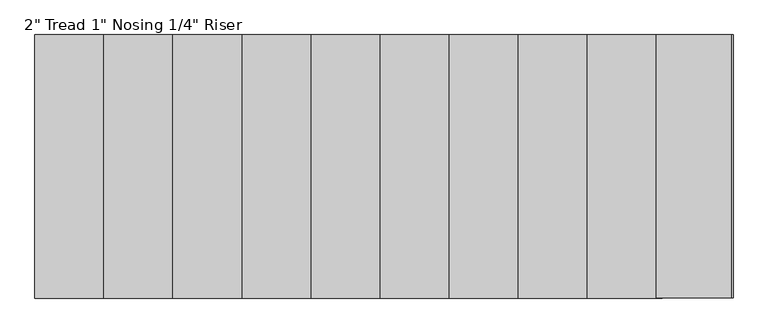
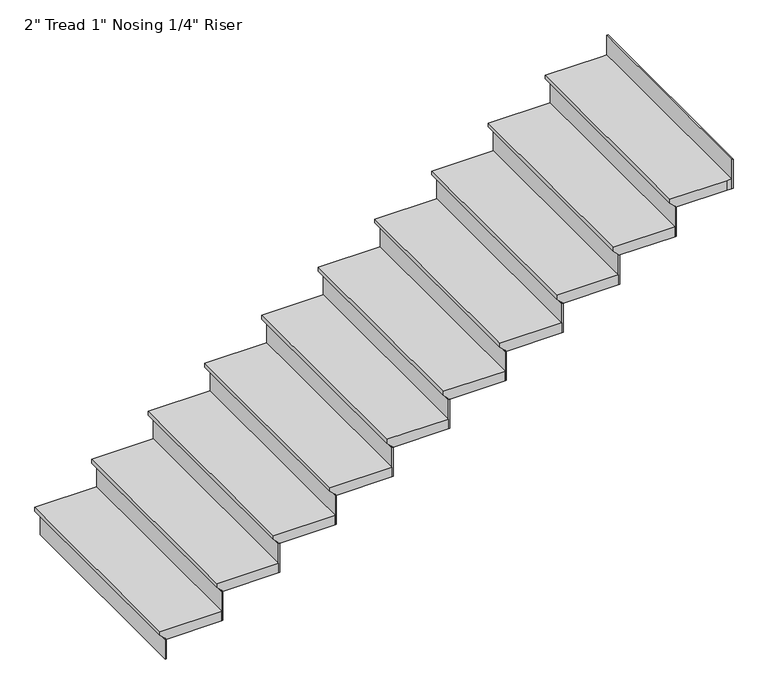
"""IFC4 building model written with IfcOpenShell, lengths in millimetres: stair flight geometry."""

from ifc_helpers import new_model, si_unit, origin, place, context, project, spatial, faceted_brep, source, transform, mapped, element, save


def stair_flight_2c29bb35(model_context):
    return source(origin(), model_context, "Body", "Brep", [
        faceted_brep([(-459.26646, -1849.1834702, 3181.35), (-459.26646, -1849.1834702, 3200.4), (-459.26646, -782.3834702, 3200.4), (-459.26646, -782.3834702, 3181.35), (-433.86646, -1849.1834702, 3155.95), (-433.86646, -782.3834702, 3155.95), (-154.46646, -1849.1834702, 3200.4), (-154.46646, -782.3834702, 3200.4), (-433.86646, -782.3834702, 3149.6), (-154.46646, -782.3834702, 3149.6), (-154.46646, -1849.1834702, 3149.6), (-433.86646, -1849.1834702, 3149.6)], [[[0, 1, 2, 3]], [[4, 0, 3, 5]], [[2, 1, 6, 7]], [[8, 9, 10, 11]], [[2, 7, 9, 8, 5, 3]], [[8, 11, 4, 5]], [[6, 1, 0, 4, 11, 10]], [[7, 6, 10, 9]]]),
        faceted_brep([(-433.86646, -1849.1834702, 3149.6), (-433.86646, -1849.1834702, 3048.0), (-427.51646, -1849.1834702, 3048.0), (-427.51646, -1849.1834702, 3149.6), (-433.86646, -782.3834702, 3149.6), (-427.51646, -782.3834702, 3149.6), (-427.51646, -782.3834702, 3048.0), (-433.86646, -782.3834702, 3048.0)], [[[0, 1, 2, 3]], [[4, 5, 6, 7]], [[1, 0, 4, 7]], [[2, 1, 7, 6]], [[3, 2, 6, 5]], [[0, 3, 5, 4]]]),
        faceted_brep([(-154.46646, -1849.1834702, 3302.0), (-154.46646, -1849.1834702, 3149.6), (-148.11646, -1849.1834702, 3149.6), (-148.11646, -1849.1834702, 3302.0), (-154.46646, -782.3834702, 3302.0), (-148.11646, -782.3834702, 3302.0), (-148.11646, -782.3834702, 3149.6), (-154.46646, -782.3834702, 3149.6)], [[[0, 1, 2, 3]], [[4, 5, 6, 7]], [[1, 0, 4, 7]], [[2, 1, 7, 6]], [[3, 2, 6, 5]], [[0, 3, 5, 4]]]),
        faceted_brep([(-179.86646, -782.3834702, 3352.8), (-179.86646, -1849.1834702, 3352.8), (124.93354, -1849.1834702, 3352.8), (124.93354, -782.3834702, 3352.8), (-154.46646, -782.3834702, 3302.0), (124.93354, -782.3834702, 3302.0), (124.93354, -1849.1834702, 3302.0), (-154.46646, -1849.1834702, 3302.0), (-154.46646, -782.3834702, 3308.35), (-179.86646, -782.3834702, 3333.75), (-154.46646, -1849.1834702, 3308.35), (-179.86646, -1849.1834702, 3333.75)], [[[0, 1, 2, 3]], [[4, 5, 6, 7]], [[0, 3, 5, 4, 8, 9]], [[4, 7, 10, 8]], [[2, 1, 11, 10, 7, 6]], [[3, 2, 6, 5]], [[11, 1, 0, 9]], [[10, 11, 9, 8]]]),
        faceted_brep([(124.93354, -1849.1834702, 3454.4), (124.93354, -1849.1834702, 3302.0), (131.28354, -1849.1834702, 3302.0), (131.28354, -1849.1834702, 3454.4), (124.93354, -782.3834702, 3454.4), (131.28354, -782.3834702, 3454.4), (131.28354, -782.3834702, 3302.0), (124.93354, -782.3834702, 3302.0)], [[[0, 1, 2, 3]], [[4, 5, 6, 7]], [[1, 0, 4, 7]], [[2, 1, 7, 6]], [[3, 2, 6, 5]], [[0, 3, 5, 4]]]),
        faceted_brep([(99.53354, -782.3834702, 3505.2), (99.53354, -1849.1834702, 3505.2), (404.33354, -1849.1834702, 3505.2), (404.33354, -782.3834702, 3505.2), (124.93354, -782.3834702, 3454.4), (404.33354, -782.3834702, 3454.4), (404.33354, -1849.1834702, 3454.4), (124.93354, -1849.1834702, 3454.4), (124.93354, -782.3834702, 3460.75), (99.53354, -782.3834702, 3486.15), (124.93354, -1849.1834702, 3460.75), (99.53354, -1849.1834702, 3486.15)], [[[0, 1, 2, 3]], [[4, 5, 6, 7]], [[0, 3, 5, 4, 8, 9]], [[4, 7, 10, 8]], [[2, 1, 11, 10, 7, 6]], [[3, 2, 6, 5]], [[11, 1, 0, 9]], [[10, 11, 9, 8]]]),
        faceted_brep([(404.33354, -1849.1834702, 3606.8), (404.33354, -1849.1834702, 3454.4), (410.68354, -1849.1834702, 3454.4), (410.68354, -1849.1834702, 3606.8), (404.33354, -782.3834702, 3606.8), (410.68354, -782.3834702, 3606.8), (410.68354, -782.3834702, 3454.4), (404.33354, -782.3834702, 3454.4)], [[[0, 1, 2, 3]], [[4, 5, 6, 7]], [[1, 0, 4, 7]], [[2, 1, 7, 6]], [[3, 2, 6, 5]], [[0, 3, 5, 4]]]),
        faceted_brep([(378.93354, -782.3834702, 3657.6), (378.93354, -1849.1834702, 3657.6), (683.73354, -1849.1834702, 3657.6), (683.73354, -782.3834702, 3657.6), (404.33354, -782.3834702, 3606.8), (683.73354, -782.3834702, 3606.8), (683.73354, -1849.1834702, 3606.8), (404.33354, -1849.1834702, 3606.8), (404.33354, -782.3834702, 3613.15), (378.93354, -782.3834702, 3638.55), (404.33354, -1849.1834702, 3613.15), (378.93354, -1849.1834702, 3638.55)], [[[0, 1, 2, 3]], [[4, 5, 6, 7]], [[0, 3, 5, 4, 8, 9]], [[4, 7, 10, 8]], [[2, 1, 11, 10, 7, 6]], [[3, 2, 6, 5]], [[11, 1, 0, 9]], [[10, 11, 9, 8]]]),
        faceted_brep([(683.73354, -1849.1834702, 3759.2), (683.73354, -1849.1834702, 3606.8), (690.08354, -1849.1834702, 3606.8), (690.08354, -1849.1834702, 3759.2), (683.73354, -782.3834702, 3759.2), (690.08354, -782.3834702, 3759.2), (690.08354, -782.3834702, 3606.8), (683.73354, -782.3834702, 3606.8)], [[[0, 1, 2, 3]], [[4, 5, 6, 7]], [[1, 0, 4, 7]], [[2, 1, 7, 6]], [[3, 2, 6, 5]], [[0, 3, 5, 4]]]),
        faceted_brep([(658.33354, -782.3834702, 3810.0), (658.33354, -1849.1834702, 3810.0), (963.13354, -1849.1834702, 3810.0), (963.13354, -782.3834702, 3810.0), (683.73354, -782.3834702, 3759.2), (963.13354, -782.3834702, 3759.2), (963.13354, -1849.1834702, 3759.2), (683.73354, -1849.1834702, 3759.2), (683.73354, -782.3834702, 3765.55), (658.33354, -782.3834702, 3790.95), (683.73354, -1849.1834702, 3765.55), (658.33354, -1849.1834702, 3790.95)], [[[0, 1, 2, 3]], [[4, 5, 6, 7]], [[0, 3, 5, 4, 8, 9]], [[4, 7, 10, 8]], [[2, 1, 11, 10, 7, 6]], [[3, 2, 6, 5]], [[11, 1, 0, 9]], [[10, 11, 9, 8]]]),
        faceted_brep([(963.13354, -1849.1834702, 3911.6), (963.13354, -1849.1834702, 3759.2), (969.48354, -1849.1834702, 3759.2), (969.48354, -1849.1834702, 3911.6), (963.13354, -782.3834702, 3911.6), (969.48354, -782.3834702, 3911.6), (969.48354, -782.3834702, 3759.2), (963.13354, -782.3834702, 3759.2)], [[[0, 1, 2, 3]], [[4, 5, 6, 7]], [[1, 0, 4, 7]], [[2, 1, 7, 6]], [[3, 2, 6, 5]], [[0, 3, 5, 4]]]),
        faceted_brep([(937.73354, -782.3834702, 3962.4), (937.73354, -1849.1834702, 3962.4), (1242.53354, -1849.1834702, 3962.4), (1242.53354, -782.3834702, 3962.4), (963.13354, -782.3834702, 3911.6), (1242.53354, -782.3834702, 3911.6), (1242.53354, -1849.1834702, 3911.6), (963.13354, -1849.1834702, 3911.6), (963.13354, -782.3834702, 3917.95), (937.73354, -782.3834702, 3943.35), (963.13354, -1849.1834702, 3917.95), (937.73354, -1849.1834702, 3943.35)], [[[0, 1, 2, 3]], [[4, 5, 6, 7]], [[0, 3, 5, 4, 8, 9]], [[4, 7, 10, 8]], [[2, 1, 11, 10, 7, 6]], [[3, 2, 6, 5]], [[11, 1, 0, 9]], [[10, 11, 9, 8]]]),
        faceted_brep([(1242.53354, -1849.1834702, 4064.0), (1242.53354, -1849.1834702, 3911.6), (1248.88354, -1849.1834702, 3911.6), (1248.88354, -1849.1834702, 4064.0), (1242.53354, -782.3834702, 4064.0), (1248.88354, -782.3834702, 4064.0), (1248.88354, -782.3834702, 3911.6), (1242.53354, -782.3834702, 3911.6)], [[[0, 1, 2, 3]], [[4, 5, 6, 7]], [[1, 0, 4, 7]], [[2, 1, 7, 6]], [[3, 2, 6, 5]], [[0, 3, 5, 4]]]),
        faceted_brep([(1217.13354, -782.3834702, 4114.8), (1217.13354, -1849.1834702, 4114.8), (1521.93354, -1849.1834702, 4114.8), (1521.93354, -782.3834702, 4114.8), (1242.53354, -782.3834702, 4064.0), (1521.93354, -782.3834702, 4064.0), (1521.93354, -1849.1834702, 4064.0), (1242.53354, -1849.1834702, 4064.0), (1242.53354, -782.3834702, 4070.35), (1217.13354, -782.3834702, 4095.75), (1242.53354, -1849.1834702, 4070.35), (1217.13354, -1849.1834702, 4095.75)], [[[0, 1, 2, 3]], [[4, 5, 6, 7]], [[0, 3, 5, 4, 8, 9]], [[4, 7, 10, 8]], [[2, 1, 11, 10, 7, 6]], [[3, 2, 6, 5]], [[11, 1, 0, 9]], [[10, 11, 9, 8]]]),
        faceted_brep([(1521.93354, -1849.1834702, 4216.4), (1521.93354, -1849.1834702, 4064.0), (1528.28354, -1849.1834702, 4064.0), (1528.28354, -1849.1834702, 4216.4), (1521.93354, -782.3834702, 4216.4), (1528.28354, -782.3834702, 4216.4), (1528.28354, -782.3834702, 4064.0), (1521.93354, -782.3834702, 4064.0)], [[[0, 1, 2, 3]], [[4, 5, 6, 7]], [[1, 0, 4, 7]], [[2, 1, 7, 6]], [[3, 2, 6, 5]], [[0, 3, 5, 4]]]),
        faceted_brep([(1496.53354, -782.3834702, 4267.2), (1496.53354, -1849.1834702, 4267.2), (1801.33354, -1849.1834702, 4267.2), (1801.33354, -782.3834702, 4267.2), (1521.93354, -782.3834702, 4216.4), (1801.33354, -782.3834702, 4216.4), (1801.33354, -1849.1834702, 4216.4), (1521.93354, -1849.1834702, 4216.4), (1521.93354, -782.3834702, 4222.75), (1496.53354, -782.3834702, 4248.15), (1521.93354, -1849.1834702, 4222.75), (1496.53354, -1849.1834702, 4248.15)], [[[0, 1, 2, 3]], [[4, 5, 6, 7]], [[0, 3, 5, 4, 8, 9]], [[4, 7, 10, 8]], [[2, 1, 11, 10, 7, 6]], [[3, 2, 6, 5]], [[11, 1, 0, 9]], [[10, 11, 9, 8]]]),
        faceted_brep([(1801.33354, -1849.1834702, 4368.8), (1801.33354, -1849.1834702, 4216.4), (1807.68354, -1849.1834702, 4216.4), (1807.68354, -1849.1834702, 4368.8), (1801.33354, -782.3834702, 4368.8), (1807.68354, -782.3834702, 4368.8), (1807.68354, -782.3834702, 4216.4), (1801.33354, -782.3834702, 4216.4)], [[[0, 1, 2, 3]], [[4, 5, 6, 7]], [[1, 0, 4, 7]], [[2, 1, 7, 6]], [[3, 2, 6, 5]], [[0, 3, 5, 4]]]),
        faceted_brep([(1775.93354, -782.3834702, 4419.6), (1775.93354, -1849.1834702, 4419.6), (2080.73354, -1849.1834702, 4419.6), (2080.73354, -782.3834702, 4419.6), (1801.33354, -782.3834702, 4368.8), (2080.73354, -782.3834702, 4368.8), (2080.73354, -1849.1834702, 4368.8), (1801.33354, -1849.1834702, 4368.8), (1801.33354, -782.3834702, 4375.15), (1775.93354, -782.3834702, 4400.55), (1801.33354, -1849.1834702, 4375.15), (1775.93354, -1849.1834702, 4400.55)], [[[0, 1, 2, 3]], [[4, 5, 6, 7]], [[0, 3, 5, 4, 8, 9]], [[4, 7, 10, 8]], [[2, 1, 11, 10, 7, 6]], [[3, 2, 6, 5]], [[11, 1, 0, 9]], [[10, 11, 9, 8]]]),
        faceted_brep([(2360.13354, -1849.1834702, 4673.6), (2360.13354, -1849.1834702, 4521.2), (2366.48354, -1849.1834702, 4521.2), (2366.48354, -1849.1834702, 4673.6), (2360.13354, -782.3834702, 4673.6), (2366.48354, -782.3834702, 4673.6), (2366.48354, -782.3834702, 4521.2), (2360.13354, -782.3834702, 4521.2)], [[[0, 1, 2, 3]], [[4, 5, 6, 7]], [[1, 0, 4, 7]], [[2, 1, 7, 6]], [[3, 2, 6, 5]], [[0, 3, 5, 4]]]),
        faceted_brep([(2080.73354, -1849.1834702, 4521.2), (2080.73354, -1849.1834702, 4368.8), (2087.08354, -1849.1834702, 4368.8), (2087.08354, -1849.1834702, 4521.2), (2080.73354, -782.3834702, 4521.2), (2087.08354, -782.3834702, 4521.2), (2087.08354, -782.3834702, 4368.8), (2080.73354, -782.3834702, 4368.8)], [[[0, 1, 2, 3]], [[4, 5, 6, 7]], [[1, 0, 4, 7]], [[2, 1, 7, 6]], [[3, 2, 6, 5]], [[0, 3, 5, 4]]]),
        faceted_brep([(2360.13354, -782.3834702, 4572.0), (2334.73354, -782.3834702, 4572.0), (2055.33354, -782.3834702, 4572.0), (2055.33354, -1849.1834702, 4572.0), (2334.73354, -1849.1834702, 4572.0), (2360.13354, -1849.1834702, 4572.0), (2334.73354, -782.3834702, 4521.2), (2360.13354, -782.3834702, 4521.2), (2360.13354, -1849.1834702, 4521.2), (2334.73354, -1849.1834702, 4521.2), (2080.73354, -1849.1834702, 4521.2), (2080.73354, -782.3834702, 4521.2), (2080.73354, -782.3834702, 4527.55), (2055.33354, -782.3834702, 4552.95), (2080.73354, -1849.1834702, 4527.55), (2055.33354, -1849.1834702, 4552.95)], [[[0, 1, 2, 3, 4, 5]], [[6, 7, 8, 9, 10, 11]], [[1, 0, 7, 6]], [[2, 1, 6, 11, 12, 13]], [[11, 10, 14, 12]], [[4, 3, 15, 14, 10, 9]], [[5, 4, 9, 8]], [[0, 5, 8, 7]], [[15, 3, 2, 13]], [[14, 15, 13, 12]]]),
    ])


if __name__ == "__main__":
    model = new_model("IFC4")
    model_context = context("Model", 3, world=origin())
    ifc_project = project(units=[si_unit("LENGTHUNIT", "METRE", prefix="MILLI")], contexts=[model_context])
    site = spatial("IfcSite", under=ifc_project)
    building = spatial("IfcBuilding", under=site)
    placement = place(None, origin())
    stair_flight_shape = stair_flight_2c29bb35(model_context)
    element("IfcStairFlight", 1, ObjectType="2\" Tread 1\" Nosing 1/4\" Riser", at=placement, inside=building, context=model_context, shape_type="MappedRepresentation", body=[
        mapped(stair_flight_shape, transform((0.0, 0.0, 0.0), x_axis=(1.0, 0.0, 0.0), y_axis=(0.0, 1.0, 0.0), z_axis=(0.0, 0.0, 1.0))),
    ])
    save(model, "model.ifc")
